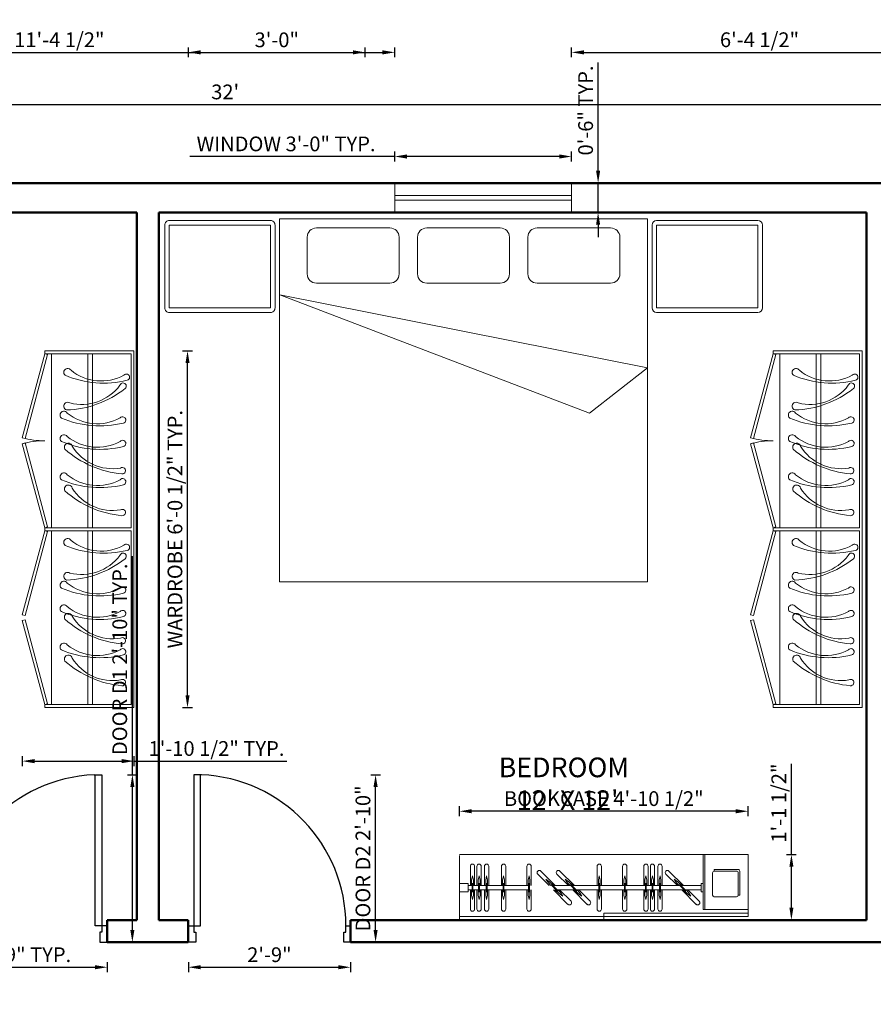
# Model space of a CAD drawing. Units: inches. Extents: x 1961 to 3038, y 800 to 1438.
# Tile 12 of 13: x 2775 to 2949, y 1148 to 1348. Entities that reach past the tile are written whole.
import ezdxf

# ---------------------------------------------------------------- set-up
doc = ezdxf.new("R2010")
doc.units = ezdxf.units.IN
for name, color, linetype, lineweight in [('A-ANNO-DIMS', 2, 'Continuous', 18), ('A-AREA-IDEN', 7, 'Continuous', 25), ('A-DOOR', 3, 'Continuous', 25), ('A-FURN', 8, 'Continuous', 18), ('A-GLAZ', 4, 'Continuous', 18), ('A-WALL', 7, 'Continuous', 50)]:
    doc.layers.add(name, color=color, linetype=linetype, lineweight=lineweight)
doc.styles.get("Standard").update_dxf_attribs({"font": 'arial.ttf'})
doc.dimstyles.new('ISO-25', dxfattribs={"dimtxt": 3, "dimasz": 2.5, "dimexe": 1, "dimexo": 1, "dimtad": 1, "dimdec": 4, "dimlunit": 4, "dimtxsty": 'Standard', "dimcen": 2.5, "dimadec": 0, "dimazin": 0, "dimtfac": 1, "dimtdec": 4, "dimtmove": 0, "dimatfit": 3, "dimfxl": 1, "dimfxlon": 1, "dimarcsym": 0})

# ---------------------------------------------------------------- blocks, each defined once
blk = doc.blocks.new('door 29')
for p, q in [((2811.91, 1194.49), (2810.4, 1194.49)), ((2810.4, 1194.49), (2810.4, 1163.76)), ((2811.74, 1163.76), (2811.74, 1194.49)), ((2809.27, 1163.76), (2811.74, 1163.76)), ((2810.4, 1163.76), (2810.4, 1162.42)), ((2810.4, 1162.42), (2810.81, 1162.42)), ((2810.81, 1162.42), (2810.81, 1160.42)), ((2810.81, 1160.42), (2809.27, 1160.42))]:
    blk.add_line(p, q)
blk.add_lwpolyline([(2842.27, 1160.42), (2840.93, 1160.42), (2840.93, 1162.42), (2841.34, 1162.42), (2841.34, 1163.76), (2842.27, 1163.76)])
blk.add_arc((2810.58, 1163.76), 30.76, 0, 87.5104)
blk = doc.blocks.new('A$C793B20D3')
for p, q in [((0.575, 1.9405), (0.025, 1.9405)), ((0.025, 1.9405), (0.025, 1.4905)), ((0.575, 1.4905), (0.575, 1.9405)), ((0.625, 0), (0.625, 1.975)), ((2.625, 1.975), (0.625, 1.975)), ((2.625, 0), (2.625, 1.975)), ((2.65, 1.4905), (2.65, 1.9405)), ((2.675, 1.9655), (3.225, 1.9655)), ((3.25, 1.9405), (3.25, 1.4905)), ((0.775, 1.675), (0.775, 1.875)), ((0.825, 1.925), (1.225, 1.925)), ((1.275, 1.675), (1.275, 1.875)), ((1.375, 1.675), (1.375, 1.875)), ((1.425, 1.925), (1.825, 1.925)), ((1.875, 1.675), (1.875, 1.875)), ((1.975, 1.675), (1.975, 1.875)), ((2.025, 1.925), (2.425, 1.925)), ((2.475, 1.675), (2.475, 1.875)), ((0.825, 1.625), (1.225, 1.625)), ((1.425, 1.625), (1.825, 1.625)), ((2.025, 1.625), (2.425, 1.625)), ((0.6256, 1.5604), (2.3107, 0.9169)), ((0.6256, 1.5604), (2.625, 1.1646)), ((0.025, 1.4905), (0.575, 1.4905)), ((3.225, 1.4655), (2.675, 1.4655)), ((2.3107, 0.9169), (2.625, 1.1646)), ((2.625, 0), (0.625, 0))]:
    blk.add_line(p, q)
at = {"flags": 128}
blk.add_lwpolyline([(0, 1.9405), (0, 1.4905, 0.414214), (0.025, 1.4655), (0.575, 1.4655, 0.414214), (0.6, 1.4905), (0.6, 1.9405, 0.414214), (0.575, 1.9655), (0.025, 1.9655, 0.414214)], format="xyb", close=True, dxfattribs=at)
blk.add_lwpolyline([(3.225, 1.9405), (3.225, 1.4905), (2.675, 1.4905), (2.675, 1.9405)], close=True)
for centre, radius, start, end in [((2.675, 1.9405), 0.025, 90, 180), ((3.225, 1.9405), 0.025, 0, 90), ((0.825, 1.875), 0.05, 90, 180), ((1.225, 1.875), 0.05, 0, 90), ((1.425, 1.875), 0.05, 90, 180), ((1.825, 1.875), 0.05, 0, 90), ((2.025, 1.875), 0.05, 90, 180), ((2.425, 1.875), 0.05, 0, 90), ((0.825, 1.675), 0.05, 180, 270), ((1.225, 1.675), 0.05, 270, 0), ((1.425, 1.675), 0.05, 180, 270), ((1.825, 1.675), 0.05, 270, 0), ((2.025, 1.675), 0.05, 180, 270), ((2.425, 1.675), 0.05, 270, 0), ((2.675, 1.4905), 0.025, 180, 270), ((3.225, 1.4905), 0.025, 270, 0)]:
    blk.add_arc(centre, radius, start, end)
blk = doc.blocks.new('A$C41DA168A')
for p, q in [((151.4, 2380), (151.4, 2400)), ((151.4, 2400), (751.4, 2400)), ((751.4, 2400), (751.4, 0)), ((151.4, 2380), (0, 1814.9)), ((19.3, 1809.8), (170.7, 2374.8)), ((731.4, 2380), (151.4, 2380)), ((170.7, 2374.8), (151.4, 2380)), ((196.6, 1210), (196.6, 2380)), ((441.4, 1210), (441.4, 2380)), ((471.4, 1210), (471.4, 2380)), ((731.4, 1210), (731.4, 2380)), ((0, 1814.9), (19.3, 1809.8)), ((0, 1775.1), (19.3, 1780.2)), ((151.4, 1210), (0, 1775.1)), ((19.3, 1780.2), (170.7, 1215.2)), ((170.7, 1215.2), (151.4, 1210)), ((151.4, 1210), (731.4, 1210)), ((151.4, 1190), (151.4, 1210)), ((151.4, 1190), (0, 624.9)), ((19.3, 619.8), (170.7, 1184.8)), ((731.4, 1190), (151.4, 1190)), ((170.7, 1184.8), (151.4, 1190)), ((196.6, 20), (196.6, 1190)), ((441.4, 1190), (441.4, 20)), ((471.4, 1190), (471.4, 20)), ((731.4, 20), (731.4, 1190)), ((0, 624.9), (19.3, 619.8)), ((0, 585.1), (19.3, 590.2)), ((151.4, 20), (0, 585.1)), ((19.3, 590.2), (170.7, 25.2)), ((170.7, 25.2), (151.4, 20)), ((151.4, 0), (151.4, 20)), ((151.4, 20), (731.4, 20)), ((751.4, 0), (151.4, 0))]:
    blk.add_line(p, q)
for centre, radius, start, end in [((305.7, 2255.1), 26.3, 32.27517, 228.96506), ((530.9, 2518.7), 321.7, 230.8748, 298.39865), ((548.2, 2849.7), 667, 247.08357, 283.63935), ((700.5, 2222.3), 21.4, 283.29422, 141.17028), ((277.3, 2668.9), 667, 271.7885, 308.34429), ((399.9, 2361), 321.7, 255.57974, 323.10358), ((677.9, 2162.6), 21.4, 307.99916, 165.87521), ((305.5, 2027.4), 26.3, 56.9801, 253.67), ((280.2, 1967.6), 26.3, 32.27517, 228.96506), ((522.6, 2562.2), 667, 247.08357, 283.63935), ((505.3, 2231.2), 321.7, 230.8748, 298.39865), ((675, 1934.8), 21.4, 283.29422, 141.17028), ((151.4, 2380), 585, 255, 270), ((151.4, 1210), 585, 90, 105), ((280.2, 1809.7), 26.3, 32.27517, 228.96506), ((522.6, 2404.2), 667, 247.08357, 283.63935), ((505.3, 2073.2), 321.7, 230.8748, 298.39865), ((675, 1776.9), 21.4, 283.29422, 141.17028), ((309.6, 1752), 26.3, 13.45499, 210.14489), ((730.9, 2236.5), 667, 228.26339, 264.81917), ((607.8, 1928.8), 321.7, 212.05463, 279.57847), ((672.7, 1593.6), 21.4, 264.47404, 122.3501), ((280.2, 1552.2), 26.3, 32.27517, 228.96506), ((522.6, 2146.7), 667, 247.08357, 283.63935), ((505.3, 1815.7), 321.7, 230.8748, 298.39865), ((675, 1519.4), 21.4, 283.29422, 141.17028), ((309.6, 1470.8), 26.3, 13.45499, 210.14489), ((730.9, 1955.3), 667, 228.26339, 264.81917), ((607.8, 1647.6), 321.7, 212.05463, 279.57847), ((672.7, 1312.3), 21.4, 264.47404, 122.3501), ((305.7, 1111), 26.3, 32.27517, 228.96506), ((548.2, 1705.5), 667, 247.08357, 283.63935), ((530.9, 1374.6), 321.7, 230.8748, 298.39865), ((700.5, 1078.2), 21.4, 283.29422, 141.17028), ((277.3, 1524.8), 667, 271.7885, 308.34429), ((399.9, 1216.9), 321.7, 255.57974, 323.10358), ((677.9, 1018.5), 21.4, 307.99916, 165.87521), ((305.5, 883.3), 26.3, 56.9801, 253.67), ((280.2, 823.5), 26.3, 32.27517, 228.96506), ((522.6, 1418), 667, 247.08357, 283.63935), ((505.3, 1087.1), 321.7, 230.8748, 298.39865), ((675, 790.7), 21.4, 283.29422, 141.17028), ((280.2, 665.6), 26.3, 32.27517, 228.96506), ((505.3, 929.1), 321.7, 230.8748, 298.39865), ((522.6, 1260.1), 667, 247.08357, 283.63935), ((309.6, 607.9), 26.3, 13.45499, 210.14489), ((607.8, 784.7), 321.7, 212.05463, 279.57847), ((675, 632.8), 21.4, 283.29422, 141.17028), ((730.9, 1092.4), 667, 228.26339, 264.81917), ((672.7, 449.5), 21.4, 264.47404, 122.3501), ((280.2, 408.1), 26.3, 32.27517, 228.96506), ((505.3, 671.6), 321.7, 230.8748, 298.39865), ((522.6, 1002.6), 667, 247.08357, 283.63935), ((309.6, 326.7), 26.3, 13.45499, 210.14489), ((607.8, 503.5), 321.7, 212.05463, 279.57847), ((675, 375.3), 21.4, 283.29422, 141.17028), ((730.9, 811.2), 667, 228.26339, 264.81917), ((672.7, 168.2), 21.4, 264.47404, 122.3501)]:
    blk.add_arc(centre, radius, start, end)
blk = doc.blocks.new('A$C58C54B33')
for p, q in [((0, 3374), (0, 1687)), ((756, 3374), (0, 3374)), ((40, 3374), (40, 0)), ((428, 3374), (328, 3374)), ((328, 3274), (328, 3374)), ((428, 3274), (428, 3374)), ((766, 3374), (766, 0)), ((353, 3247), (128, 3247)), ((239, 3222), (289, 3233)), ((289, 3233), (353, 3233)), ((428, 3274), (328, 3274)), ((428, 3227), (328, 3227)), ((328, 3217), (328, 3227)), ((353, 3150), (353, 3274)), ((403, 3150), (403, 3274)), ((628, 3247), (403, 3247)), ((403, 3233), (467, 3233)), ((428, 3217), (428, 3227)), ((517, 3222), (467, 3233)), ((353, 3197), (128, 3197)), ((353, 3170), (128, 3170)), ((353, 3120), (128, 3120)), ((239, 3222), (289, 3211)), ((239, 3145), (289, 3156)), ((239, 3145), (289, 3134)), ((353, 3211), (289, 3211)), ((289, 3156), (353, 3156)), ((353, 3134), (289, 3134)), ((428, 3217), (328, 3217)), ((428, 3150), (328, 3150)), ((328, 3140), (328, 3150)), ((428, 3140), (328, 3140)), ((353, 3217), (353, 3150)), ((353, 3140), (353, 3062)), ((403, 3217), (403, 3150)), ((467, 3211), (403, 3211)), ((628, 3197), (403, 3197)), ((628, 3170), (403, 3170)), ((403, 3156), (467, 3156)), ((403, 3140), (403, 3062)), ((467, 3134), (403, 3134)), ((628, 3120), (403, 3120)), ((428, 3140), (428, 3150)), ((517, 3222), (467, 3211)), ((517, 3145), (467, 3156)), ((517, 3145), (467, 3134)), ((353, 3082), (128, 3082)), ((353, 3032), (128, 3032)), ((239, 3057), (289, 3068)), ((239, 3057), (289, 3046)), ((289, 3068), (353, 3068)), ((353, 3046), (289, 3046)), ((428, 3062), (328, 3062)), ((328, 3052), (328, 3062)), ((428, 3052), (328, 3052)), ((353, 3052), (353, 2864)), ((628, 3082), (403, 3082)), ((403, 3068), (467, 3068)), ((403, 3052), (403, 2864)), ((467, 3046), (403, 3046)), ((628, 3032), (403, 3032)), ((428, 3052), (428, 3062)), ((517, 3057), (467, 3068)), ((517, 3057), (467, 3046)), ((353, 2884), (128, 2884)), ((628, 2884), (403, 2884)), ((353, 2834), (128, 2834)), ((239, 2859), (289, 2870)), ((239, 2859), (289, 2848)), ((289, 2870), (353, 2870)), ((353, 2848), (289, 2848)), ((428, 2864), (328, 2864)), ((328, 2854), (328, 2864)), ((428, 2854), (328, 2854)), ((353, 2854), (353, 2566)), ((403, 2870), (467, 2870)), ((403, 2854), (403, 2566)), ((467, 2848), (403, 2848)), ((628, 2834), (403, 2834)), ((428, 2854), (428, 2864)), ((517, 2859), (467, 2870)), ((517, 2859), (467, 2848)), ((353, 2586), (128, 2586)), ((353, 2536), (128, 2536)), ((239, 2561), (289, 2572)), ((239, 2561), (289, 2550)), ((289, 2572), (353, 2572)), ((353, 2550), (289, 2550)), ((328, 2556), (328, 2566)), ((428, 2566), (328, 2566)), ((428, 2556), (328, 2556)), ((628, 2586), (403, 2586)), ((403, 2572), (467, 2572)), ((467, 2550), (403, 2550)), ((628, 2536), (403, 2536)), ((428, 2556), (428, 2566)), ((517, 2561), (467, 2572)), ((517, 2561), (467, 2550)), ((537, 2459), (403, 2325)), ((572, 2424), (403, 2254)), ((410, 2304), (339, 2233)), ((403, 2305), (433, 2335)), ((448, 2320), (403, 2274)), ((417, 2296), (410, 2304)), ((476, 2363), (433, 2335)), ((476, 2363), (448, 2320)), ((353, 2275), (183, 2106)), ((353, 2204), (219, 2070)), ((280, 2167), (308, 2210)), ((280, 2167), (323, 2194)), ((308, 2210), (353, 2255)), ((353, 2224), (323, 2194)), ((346, 2226), (339, 2233)), ((417, 2296), (346, 2226)), ((353, 2233), (353, 2022)), ((403, 2283), (403, 2072)), ((537, 2235), (403, 2101)), ((572, 2200), (403, 2030)), ((410, 2079), (339, 2009)), ((417, 2072), (346, 2002)), ((403, 2081), (433, 2111)), ((448, 2095), (403, 2050)), ((417, 2072), (410, 2079)), ((476, 2138), (433, 2111)), ((476, 2138), (448, 2095)), ((353, 2051), (183, 1881)), ((353, 1980), (219, 1846)), ((280, 1942), (308, 1985)), ((280, 1942), (323, 1970)), ((308, 1985), (353, 2031)), ((353, 2000), (323, 1970)), ((346, 2002), (339, 2009)), ((353, 1745), (353, 2008)), ((403, 1745), (403, 2058)), ((353, 1765), (128, 1765)), ((239, 1740), (289, 1751)), ((239, 1740), (289, 1729)), ((289, 1751), (353, 1751)), ((353, 1729), (289, 1729)), ((428, 1745), (328, 1745)), ((328, 1735), (328, 1745)), ((428, 1735), (328, 1735)), ((353, 1735), (353, 1447)), ((628, 1765), (403, 1765)), ((403, 1751), (467, 1751)), ((403, 1735), (403, 1447)), ((467, 1729), (403, 1729)), ((428, 1735), (428, 1745)), ((517, 1740), (467, 1751)), ((517, 1740), (467, 1729)), ((0, 1687), (80, 1687)), ((80, 1687), (80, 0)), ((353, 1715), (128, 1715)), ((628, 1715), (403, 1715)), ((353, 1467), (128, 1467)), ((353, 1417), (128, 1417)), ((239, 1442), (289, 1453)), ((239, 1442), (289, 1431)), ((289, 1453), (353, 1453)), ((353, 1431), (289, 1431)), ((328, 1437), (328, 1447)), ((428, 1447), (328, 1447)), ((428, 1437), (328, 1437)), ((353, 1123), (353, 1437)), ((628, 1467), (403, 1467)), ((403, 1453), (467, 1453)), ((403, 1123), (403, 1437)), ((467, 1431), (403, 1431)), ((628, 1417), (403, 1417)), ((428, 1437), (428, 1447)), ((517, 1442), (467, 1453)), ((517, 1442), (467, 1431)), ((353, 1220), (128, 1220)), ((353, 1170), (128, 1170)), ((239, 1195), (289, 1206)), ((239, 1195), (289, 1184)), ((289, 1206), (353, 1206)), ((353, 1184), (289, 1184)), ((428, 1200), (328, 1200)), ((328, 1190), (328, 1200)), ((428, 1190), (328, 1190)), ((353, 1190), (353, 1123)), ((628, 1220), (403, 1220)), ((403, 1206), (467, 1206)), ((403, 1190), (403, 1123)), ((467, 1184), (403, 1184)), ((628, 1170), (403, 1170)), ((428, 1190), (428, 1200)), ((517, 1195), (467, 1206)), ((517, 1195), (467, 1184)), ((353, 1143), (128, 1143)), ((353, 1093), (128, 1093)), ((353, 1055), (128, 1055)), ((239, 1118), (289, 1129)), ((239, 1118), (289, 1107)), ((239, 1030), (289, 1041)), ((289, 1129), (353, 1129)), ((353, 1107), (289, 1107)), ((289, 1041), (353, 1041)), ((428, 1123), (328, 1123)), ((328, 1113), (328, 1123)), ((428, 1113), (328, 1113)), ((353, 1113), (353, 1035)), ((628, 1143), (403, 1143)), ((403, 1129), (467, 1129)), ((403, 1113), (403, 1035)), ((467, 1107), (403, 1107)), ((628, 1093), (403, 1093)), ((628, 1055), (403, 1055)), ((403, 1041), (467, 1041)), ((428, 1113), (428, 1123)), ((517, 1118), (467, 1129)), ((517, 1118), (467, 1107)), ((517, 1030), (467, 1041)), ((353, 1005), (128, 1005)), ((239, 1030), (289, 1019)), ((353, 1019), (289, 1019)), ((428, 1035), (328, 1035)), ((328, 1025), (328, 1035)), ((428, 1025), (328, 1025)), ((353, 1025), (353, 748)), ((403, 1025), (403, 798)), ((467, 1019), (403, 1019)), ((628, 1005), (403, 1005)), ((537, 961), (403, 826)), ((572, 925), (403, 756)), ((428, 1025), (428, 1035)), ((517, 1030), (467, 1019)), ((403, 807), (433, 836)), ((448, 821), (403, 776)), ((476, 864), (433, 836)), ((476, 864), (448, 821)), ((353, 776), (183, 607)), ((353, 706), (219, 572)), ((280, 668), (308, 711)), ((280, 668), (323, 696)), ((308, 711), (353, 757)), ((353, 726), (323, 696)), ((410, 805), (339, 734)), ((346, 727), (339, 734)), ((417, 798), (346, 727)), ((353, 550), (353, 734)), ((403, 550), (403, 784)), ((417, 798), (410, 805)), ((766, 525), (123, 525)), ((123, 525), (123, 0)), ((766, 505), (123, 505)), ((428, 550), (328, 550)), ((328, 550), (328, 525)), ((428, 550), (428, 525)), ((272, 136), (272, 396)), ((292, 416), (552, 416)), ((572, 398), (591, 398)), ((572, 396), (572, 136)), ((591, 398), (591, 118)), ((291, 98), (291, 116)), ((552, 116), (292, 116)), ((40, 0), (766, 0)), ((571, 98), (291, 98))]:
    blk.add_line(p, q)
for centre, radius, start, end in [((128, 3222), 25, 90, 270), ((628, 3222), 25, 270, 90), ((128, 3145), 25, 90, 270), ((628, 3145), 25, 270, 90), ((128, 3057), 25, 90, 270), ((628, 3057), 25, 270, 90), ((128, 2859), 25, 90, 270), ((628, 2859), 25, 270, 90), ((128, 2561), 25, 90, 270), ((628, 2561), 25, 270, 90), ((555, 2441), 25, 315, 135), ((555, 2217), 25, 315, 135), ((201, 2088), 25, 135, 315), ((201, 1864), 25, 135, 315), ((128, 1740), 25, 90, 270), ((628, 1740), 25, 270, 90), ((128, 1442), 25, 90, 270), ((628, 1442), 25, 270, 90), ((128, 1195), 25, 90, 270), ((628, 1195), 25, 270, 90), ((128, 1118), 25, 90, 270), ((128, 1030), 25, 90, 270), ((628, 1118), 25, 270, 90), ((628, 1030), 25, 270, 90), ((555, 943), 25, 315, 135), ((201, 589), 25, 135, 315), ((292, 396), 20, 90, 180), ((552, 396), 20, 0, 90), ((292, 136), 20, 180, 270), ((552, 136), 20, 270, 0), ((571, 118), 20, 270, 0)]:
    blk.add_arc(centre, radius, start, end)
blk = doc.blocks.new('*D25')
at = {"layer": 'A-ANNO-DIMS', "color": 0, "lineweight": -2, "transparency": 16777216}
for p, q in [((2624.77, 1329.92), (2624.77, 1331.92)), ((2627.27, 1330.92), (3006.27, 1330.92)), ((3008.77, 1329.92), (3008.77, 1331.92))]:
    blk.add_line(p, q, dxfattribs=at)
at = {"layer": 'A-ANNO-DIMS', "color": 0, "transparency": 16777216}
for points in [[(2627.27, 1331.34), (2627.27, 1330.51), (2624.77, 1330.92)], [(3006.27, 1331.34), (3006.27, 1330.51), (3008.77, 1330.92)]]:
    blk.add_solid(points, dxfattribs=at)
at = {"layer": 'Defpoints', "color": 0, "transparency": 16777216}
for p in [(3008.77, 1330.92), (2624.77, 1314.92), (3008.77, 1314.92)]:
    blk.add_point(p, dxfattribs=at)
at = {"layer": 'A-ANNO-DIMS', "color": 0, "transparency": 16777216, "insert": (2816.77, 1333.08), "char_height": 3, "attachment_point": 5}
blk.add_mtext("32'", dxfattribs=at)
blk = doc.blocks.new('WIN-36IN')
for p, q in [((0, 36), (6, 36)), ((2.5, 36), (2.5, 0)), ((3.5, 36), (3.5, 0)), ((0, 0), (6, 0))]:
    blk.add_line(p, q)
blk = doc.blocks.new('DOOR-SWING-33IN')
for p, q in [((30.36, 34.07), (31.87, 34.07)), ((30.53, 3.34), (30.53, 34.07)), ((31.87, 34.07), (31.87, 3.34)), ((33, 3.34), (30.53, 3.34)), ((31.87, 2), (31.46, 2)), ((31.46, 2), (31.46, 0)), ((31.87, 3.34), (31.87, 2)), ((31.46, 0), (33, 0))]:
    blk.add_line(p, q)
blk.add_lwpolyline([(0, 0), (1.34, 0), (1.34, 2), (0.93, 2), (0.93, 3.34), (0, 3.34)])
blk.add_arc((31.69, 3.34), 30.76, 92.4896, 180)
blk = doc.blocks.new('*D31')
at = {"layer": 'A-ANNO-DIMS', "color": 0, "lineweight": -2, "transparency": 16777216}
for p, q in [((2808.1, 1280.77), (2810.1, 1280.77)), ((2809.1, 1210.65), (2809.1, 1278.27)), ((2808.1, 1208.15), (2810.1, 1208.15))]:
    blk.add_line(p, q, dxfattribs=at)
at = {"layer": 'A-ANNO-DIMS', "color": 0, "transparency": 16777216}
for points in [[(2808.69, 1278.27), (2809.52, 1278.27), (2809.1, 1280.77)], [(2808.69, 1210.65), (2809.52, 1210.65), (2809.1, 1208.15)]]:
    blk.add_solid(points, dxfattribs=at)
at = {"layer": 'Defpoints', "color": 0, "transparency": 16777216}
for p in [(2798.21, 1280.77), (2809.1, 1280.77), (2798.21, 1208.15)]:
    blk.add_point(p, dxfattribs=at)
at = {"layer": 'A-ANNO-DIMS', "color": 0, "transparency": 16777216, "insert": (2806.93, 1244.46), "char_height": 3, "attachment_point": 5, "rotation": 90}
blk.add_mtext('WARDROBE 6\'-0 1/2" TYP.', dxfattribs=at)
blk = doc.blocks.new('*D32')
at = {"layer": 'A-ANNO-DIMS', "color": 0, "lineweight": -2, "transparency": 16777216}
for p, q in [((2775.47, 1198.26), (2775.47, 1196.26)), ((2777.97, 1197.26), (2795.71, 1197.26)), ((2798.21, 1198.26), (2798.21, 1196.26)), ((2798.21, 1197.26), (2829.29, 1197.26))]:
    blk.add_line(p, q, dxfattribs=at)
at = {"layer": 'A-ANNO-DIMS', "color": 0, "transparency": 16777216}
for points in [[(2777.97, 1197.68), (2777.97, 1196.84), (2775.47, 1197.26)], [(2795.71, 1197.68), (2795.71, 1196.84), (2798.21, 1197.26)]]:
    blk.add_solid(points, dxfattribs=at)
at = {"layer": 'Defpoints', "color": 0, "transparency": 16777216}
for p in [(2775.47, 1208.15), (2798.21, 1208.15), (2798.21, 1197.26)]:
    blk.add_point(p, dxfattribs=at)
at = {"layer": 'A-ANNO-DIMS', "color": 0, "transparency": 16777216, "insert": (2815, 1199.44), "char_height": 3, "attachment_point": 5}
blk.add_mtext('1\'-10 1/2" TYP.', dxfattribs=at)
blk = doc.blocks.new('*D33')
at = {"layer": 'A-ANNO-DIMS', "color": 0, "lineweight": -2, "transparency": 16777216}
for p, q in [((2851.27, 1319.32), (2851.27, 1321.32)), ((2887.27, 1319.32), (2887.27, 1321.32)), ((2851.27, 1320.32), (2809.56, 1320.32)), ((2884.77, 1320.32), (2853.77, 1320.32))]:
    blk.add_line(p, q, dxfattribs=at)
at = {"layer": 'A-ANNO-DIMS', "color": 0, "transparency": 16777216}
for points in [[(2853.77, 1320.74), (2853.77, 1319.9), (2851.27, 1320.32)], [(2884.77, 1320.74), (2884.77, 1319.9), (2887.27, 1320.32)]]:
    blk.add_solid(points, dxfattribs=at)
at = {"layer": 'Defpoints', "color": 0, "transparency": 16777216}
for p in [(2851.27, 1320.32), (2851.27, 1314.92), (2887.27, 1314.92)]:
    blk.add_point(p, dxfattribs=at)
at = {"layer": 'A-ANNO-DIMS', "color": 0, "transparency": 16777216, "insert": (2829.16, 1322.5), "char_height": 3, "attachment_point": 5}
blk.add_mtext('WINDOW 3\'-0" TYP.', dxfattribs=at)
blk = doc.blocks.new('*D34')
at = {"layer": 'A-ANNO-DIMS', "color": 0, "lineweight": -2, "transparency": 16777216}
for p, q in [((2892.67, 1317.42), (2892.67, 1339.46)), ((2891.67, 1314.92), (2893.67, 1314.92)), ((2892.67, 1308.92), (2892.67, 1314.92)), ((2891.67, 1308.92), (2893.67, 1308.92)), ((2892.67, 1306.42), (2892.67, 1303.92))]:
    blk.add_line(p, q, dxfattribs=at)
at = {"layer": 'A-ANNO-DIMS', "color": 0, "transparency": 16777216}
for points in [[(2892.25, 1317.42), (2893.08, 1317.42), (2892.67, 1314.92)], [(2892.25, 1306.42), (2893.08, 1306.42), (2892.67, 1308.92)]]:
    blk.add_solid(points, dxfattribs=at)
at = {"layer": 'Defpoints', "color": 0, "transparency": 16777216}
for p in [(2887.27, 1314.92), (2892.67, 1314.92), (2887.27, 1308.92)]:
    blk.add_point(p, dxfattribs=at)
at = {"layer": 'A-ANNO-DIMS', "color": 0, "transparency": 16777216, "insert": (2890.51, 1329.69), "char_height": 3, "attachment_point": 5, "rotation": 90}
blk.add_mtext('0\'-6" TYP.', dxfattribs=at)
blk = doc.blocks.new('*D47')
at = {"layer": 'A-ANNO-DIMS', "color": 0, "lineweight": -2, "transparency": 16777216}
for p, q in [((2797.88, 1194.49), (2797.88, 1238.97)), ((2796.88, 1194.49), (2798.88, 1194.49)), ((2797.88, 1162.92), (2797.88, 1191.99)), ((2796.88, 1160.42), (2798.88, 1160.42))]:
    blk.add_line(p, q, dxfattribs=at)
at = {"layer": 'A-ANNO-DIMS', "color": 0, "transparency": 16777216}
for points in [[(2797.46, 1191.99), (2798.3, 1191.99), (2797.88, 1194.49)], [(2797.46, 1162.92), (2798.3, 1162.92), (2797.88, 1160.42)]]:
    blk.add_solid(points, dxfattribs=at)
at = {"layer": 'Defpoints', "color": 0, "transparency": 16777216}
for p in [(2792.77, 1194.49), (2797.88, 1194.49), (2792.77, 1160.42)]:
    blk.add_point(p, dxfattribs=at)
at = {"layer": 'A-ANNO-DIMS', "color": 0, "transparency": 16777216, "insert": (2795.7, 1217.98), "char_height": 3, "attachment_point": 5, "rotation": 90}
blk.add_mtext('DOOR D1 2\'-10" TYP.', dxfattribs=at)
blk = doc.blocks.new('*D48')
at = {"layer": 'A-ANNO-DIMS', "color": 0, "lineweight": -2, "transparency": 16777216}
for p, q in [((2759.77, 1156.31), (2759.77, 1154.31)), ((2762.27, 1155.31), (2790.27, 1155.31)), ((2792.77, 1156.31), (2792.77, 1154.31))]:
    blk.add_line(p, q, dxfattribs=at)
at = {"layer": 'A-ANNO-DIMS', "color": 0, "transparency": 16777216}
for points in [[(2762.27, 1155.73), (2762.27, 1154.89), (2759.77, 1155.31)], [(2790.27, 1155.73), (2790.27, 1154.89), (2792.77, 1155.31)]]:
    blk.add_solid(points, dxfattribs=at)
at = {"layer": 'Defpoints', "color": 0, "transparency": 16777216}
for p in [(2759.77, 1160.42), (2792.77, 1160.42), (2792.77, 1155.31)]:
    blk.add_point(p, dxfattribs=at)
at = {"layer": 'A-ANNO-DIMS', "color": 0, "transparency": 16777216, "insert": (2776.27, 1157.47), "char_height": 3, "attachment_point": 5}
blk.add_mtext('2\'-9" TYP.', dxfattribs=at)
blk = doc.blocks.new('*D49')
at = {"layer": 'A-ANNO-DIMS', "color": 0, "lineweight": -2, "transparency": 16777216}
for p, q in [((2846.38, 1194.49), (2848.38, 1194.49)), ((2847.38, 1162.92), (2847.38, 1191.99)), ((2846.38, 1160.42), (2848.38, 1160.42))]:
    blk.add_line(p, q, dxfattribs=at)
at = {"layer": 'A-ANNO-DIMS', "color": 0, "transparency": 16777216}
for points in [[(2846.96, 1191.99), (2847.8, 1191.99), (2847.38, 1194.49)], [(2846.96, 1162.92), (2847.8, 1162.92), (2847.38, 1160.42)]]:
    blk.add_solid(points, dxfattribs=at)
at = {"layer": 'Defpoints', "color": 0, "transparency": 16777216}
for p in [(2842.27, 1194.49), (2847.38, 1194.49), (2842.27, 1160.42)]:
    blk.add_point(p, dxfattribs=at)
at = {"layer": 'A-ANNO-DIMS', "color": 0, "transparency": 16777216, "insert": (2845.2, 1177.46), "char_height": 3, "attachment_point": 5, "rotation": 90}
blk.add_mtext('DOOR D2 2\'-10"', dxfattribs=at)
blk = doc.blocks.new('*D50')
at = {"layer": 'A-ANNO-DIMS', "color": 0, "lineweight": -2, "transparency": 16777216}
for p, q in [((2809.27, 1156.31), (2809.27, 1154.31)), ((2811.77, 1155.31), (2839.77, 1155.31)), ((2842.27, 1156.31), (2842.27, 1154.31))]:
    blk.add_line(p, q, dxfattribs=at)
at = {"layer": 'A-ANNO-DIMS', "color": 0, "transparency": 16777216}
for points in [[(2811.77, 1155.73), (2811.77, 1154.89), (2809.27, 1155.31)], [(2839.77, 1155.73), (2839.77, 1154.89), (2842.27, 1155.31)]]:
    blk.add_solid(points, dxfattribs=at)
at = {"layer": 'Defpoints', "color": 0, "transparency": 16777216}
for p in [(2809.27, 1160.42), (2842.27, 1160.42), (2842.27, 1155.31)]:
    blk.add_point(p, dxfattribs=at)
at = {"layer": 'A-ANNO-DIMS', "color": 0, "transparency": 16777216, "insert": (2825.77, 1157.47), "char_height": 3, "attachment_point": 5}
blk.add_mtext('2\'-9"', dxfattribs=at)
blk = doc.blocks.new('*D53')
at = {"layer": 'A-ANNO-DIMS', "color": 0, "lineweight": -2, "transparency": 16777216}
for p, q in [((2864.46, 1186.06), (2864.46, 1188.06)), ((2920.7, 1187.06), (2866.96, 1187.06)), ((2923.2, 1186.06), (2923.2, 1188.06))]:
    blk.add_line(p, q, dxfattribs=at)
at = {"layer": 'A-ANNO-DIMS', "color": 0, "transparency": 16777216}
for points in [[(2866.96, 1187.48), (2866.96, 1186.64), (2864.46, 1187.06)], [(2920.7, 1187.48), (2920.7, 1186.64), (2923.2, 1187.06)]]:
    blk.add_solid(points, dxfattribs=at)
at = {"layer": 'Defpoints', "color": 0, "transparency": 16777216}
for p in [(2864.46, 1187.06), (2864.46, 1178.25), (2923.2, 1178.25)]:
    blk.add_point(p, dxfattribs=at)
at = {"layer": 'A-ANNO-DIMS', "color": 0, "transparency": 16777216, "insert": (2893.83, 1189.24), "char_height": 3, "attachment_point": 5}
blk.add_mtext('BOOKCASE 4\'-10 1/2"', dxfattribs=at)
blk = doc.blocks.new('*D54')
at = {"layer": 'A-ANNO-DIMS', "color": 0, "lineweight": -2, "transparency": 16777216}
for p, q in [((2932.01, 1178.25), (2932.01, 1196.68)), ((2931.01, 1178.25), (2933.01, 1178.25)), ((2932.01, 1167.42), (2932.01, 1175.75)), ((2931.01, 1164.92), (2933.01, 1164.92))]:
    blk.add_line(p, q, dxfattribs=at)
at = {"layer": 'A-ANNO-DIMS', "color": 0, "transparency": 16777216}
for points in [[(2931.6, 1175.75), (2932.43, 1175.75), (2932.01, 1178.25)], [(2931.6, 1167.42), (2932.43, 1167.42), (2932.01, 1164.92)]]:
    blk.add_solid(points, dxfattribs=at)
at = {"layer": 'Defpoints', "color": 0, "transparency": 16777216}
for p in [(2923.2, 1178.25), (2932.01, 1178.25), (2923.2, 1164.92)]:
    blk.add_point(p, dxfattribs=at)
at = {"layer": 'A-ANNO-DIMS', "color": 0, "transparency": 16777216, "insert": (2929.84, 1188.72), "char_height": 3, "attachment_point": 5, "rotation": 90}
blk.add_mtext('1\'-1 1/2"', dxfattribs=at)
blk = doc.blocks.new('*D75')
at = {"layer": 'A-ANNO-DIMS', "color": 0, "lineweight": -2, "transparency": 16777216}
for p, q in [((2809.27, 1340.52), (2809.27, 1342.52)), ((2811.77, 1341.52), (2842.77, 1341.52)), ((2845.27, 1340.52), (2845.27, 1342.52))]:
    blk.add_line(p, q, dxfattribs=at)
at = {"layer": 'A-ANNO-DIMS', "color": 0, "transparency": 16777216}
for points in [[(2811.77, 1341.94), (2811.77, 1341.1), (2809.27, 1341.52)], [(2842.77, 1341.94), (2842.77, 1341.1), (2845.27, 1341.52)]]:
    blk.add_solid(points, dxfattribs=at)
at = {"layer": 'Defpoints', "color": 0, "transparency": 16777216}
for p in [(2845.27, 1341.52), (2809.27, 970.92), (2845.27, 970.92)]:
    blk.add_point(p, dxfattribs=at)
at = {"layer": 'A-ANNO-DIMS', "color": 0, "transparency": 16777216, "insert": (2827.27, 1343.68), "char_height": 3, "attachment_point": 5}
blk.add_mtext('3\'-0"', dxfattribs=at)
blk = doc.blocks.new('*D77')
at = {"layer": 'A-ANNO-DIMS', "color": 0, "lineweight": -2, "transparency": 16777216}
for p, q in [((2714.77, 1340.52), (2714.77, 1342.52)), ((2717.27, 1341.52), (2848.77, 1341.52)), ((2851.27, 1340.52), (2851.27, 1342.52))]:
    blk.add_line(p, q, dxfattribs=at)
at = {"layer": 'A-ANNO-DIMS', "color": 0, "transparency": 16777216}
for points in [[(2717.27, 1341.94), (2717.27, 1341.1), (2714.77, 1341.52)], [(2848.77, 1341.94), (2848.77, 1341.1), (2851.27, 1341.52)]]:
    blk.add_solid(points, dxfattribs=at)
at = {"layer": 'Defpoints', "color": 0, "transparency": 16777216}
for p in [(2851.27, 1341.52), (2714.77, 1314.92), (2851.27, 1314.92)]:
    blk.add_point(p, dxfattribs=at)
at = {"layer": 'A-ANNO-DIMS', "color": 0, "transparency": 16777216, "insert": (2783.02, 1343.7), "char_height": 3, "attachment_point": 5}
blk.add_mtext('11\'-4 1/2"', dxfattribs=at)
blk = doc.blocks.new('*D78')
at = {"layer": 'A-ANNO-DIMS', "color": 0, "lineweight": -2, "transparency": 16777216}
for p, q in [((2887.27, 1340.52), (2887.27, 1342.52)), ((2889.77, 1341.52), (2961.27, 1341.52)), ((2963.77, 1340.52), (2963.77, 1342.52))]:
    blk.add_line(p, q, dxfattribs=at)
at = {"layer": 'A-ANNO-DIMS', "color": 0, "transparency": 16777216}
for points in [[(2889.77, 1341.94), (2889.77, 1341.1), (2887.27, 1341.52)], [(2961.27, 1341.94), (2961.27, 1341.1), (2963.77, 1341.52)]]:
    blk.add_solid(points, dxfattribs=at)
at = {"layer": 'Defpoints', "color": 0, "transparency": 16777216}
for p in [(2963.77, 1341.52), (2887.27, 1314.92), (2963.77, 1314.92)]:
    blk.add_point(p, dxfattribs=at)
at = {"layer": 'A-ANNO-DIMS', "color": 0, "transparency": 16777216, "insert": (2925.52, 1343.7), "char_height": 3, "attachment_point": 5}
blk.add_mtext('6\'-4 1/2"', dxfattribs=at)

msp = doc.modelspace()

# ---------------------------------------------------------------- linework, layer by layer
at = {"layer": 'A-WALL'}
for p, q in [((3008.76803, 1314.91975), (2624.76803, 1314.91975)), ((2798.76803, 1308.91975), (2630.76803, 1308.91975)), ((2798.76803, 1308.91975), (2798.76803, 1164.91975)), ((2803.26803, 1308.91975), (2803.26803, 1164.91975)), ((2947.26803, 1308.91975), (2803.26803, 1308.91975)), ((2947.26803, 1308.91975), (2947.26803, 1164.91975)), ((2792.76803, 1164.91975), (2792.76803, 1160.41975)), ((2798.76803, 1164.91975), (2792.76803, 1164.91975)), ((2809.26803, 1164.91975), (2803.26803, 1164.91975)), ((2809.26803, 1164.91975), (2809.26803, 1160.41975)), ((2842.26803, 1164.91975), (2842.26803, 1160.41975)), ((2947.26803, 1164.91975), (2842.26803, 1164.91975)), ((2809.26803, 1160.41975), (2792.76803, 1160.41975)), ((2957.76803, 1160.41975), (2842.26803, 1160.41975))]:
    msp.add_line(p, q, dxfattribs=at)

# ---------------------------------------------------------------- block references
at = {"layer": 'A-DOOR'}
for name, p in [('DOOR-SWING-33IN', (2759.768, 1160.42)), ('door 29', (0, 0))]:
    msp.add_blockref(name, p, dxfattribs=at)
at = {"layer": 'A-FURN'}
for name, p, xscale, yscale, zscale in [('A$C793B20D3', (2804.46147, 1233.73111), 37.42822407468409, 37.42822407468409, 37.42822407468409), ('A$C41DA168A', (2775.47468, 1208.15272), 0.0302586277246643, 0.0302586277246643, 0.0302586277246643), ('A$C41DA168A', (2923.70823, 1208.15272), 0.0302586277246643, 0.0302586277246643, 0.0302586277246643)]:
    msp.add_blockref(name, p, dxfattribs=dict(at, xscale=xscale, yscale=yscale, zscale=zscale))
at = {"layer": 'A-FURN', "xscale": 0.0174108168007704, "yscale": 0.0174108168007704, "zscale": 0.0174108168007704, "rotation": 90.0000000000012}
msp.add_blockref('A$C58C54B33', (2923.20249, 1164.91975), dxfattribs=at)
at = {"layer": 'A-GLAZ', "rotation": 90.00000000000323}
msp.add_blockref('WIN-36IN', (2887.26779, 1308.91972), dxfattribs=at)

# ---------------------------------------------------------------- texts
at = {"layer": 'A-AREA-IDEN', "insert": (2872.43492, 1197.98335), "char_height": 4, "attachment_point": 1}
msp.add_mtext_dynamic_manual_height_columns("{\\fTimes New Roman|b1|i0|c0|p18;BEDROOM\\P   12' X 12'}", width=33.1080891, gutter_width=12.5, heights=[0], dxfattribs=at)

# ---------------------------------------------------------------- dimensions: what is measured, and where the dimension line sits
at = {"layer": 'A-ANNO-DIMS'}
for base, p1, p2, override, picture, middle in [((2851.26803, 1341.51975), (2714.76803, 1314.91975), (2851.26803, 1314.91975), {"dimdec": 1, "dimlfac": 1, "dimrnd": 0, "dimzin": 1, "dimdsep": 46, "dimlunit": 4, "dimfrac": 2}, '*D77', (2783.01803, 1343.69591)), ((2963.76803, 1341.51975), (2887.26803, 1314.91975), (2963.76803, 1314.91975), {"dimdec": 1, "dimlfac": 1, "dimrnd": 0, "dimzin": 1, "dimdsep": 46, "dimlunit": 4, "dimfrac": 2}, '*D78', (2925.51803, 1343.69591)), ((2845.26803, 1341.51975), (2809.26803, 970.91975), (2845.26803, 970.91975), {"dimdec": 1, "dimlfac": 1, "dimrnd": 0, "dimzin": 1, "dimdsep": 46, "dimlunit": 4, "dimfrac": 2}, '*D75', (2827.26803, 1343.6775)), ((3008.76803, 1330.92264), (2624.76803, 1314.91975), (3008.76803, 1314.91975), {"dimclrd": 0, "dimclre": 0, "dimclrt": 0}, '*D25', (2816.76803, 1333.08038)), ((2842.26803, 1155.30859), (2809.26803, 1160.41975), (2842.26803, 1160.41975), {"dimdec": 1, "dimlfac": 1, "dimrnd": 0, "dimzin": 1, "dimdsep": 46, "dimlunit": 4, "dimfrac": 2}, '*D50', (2825.76803, 1157.46531))]:
    dim = msp.add_linear_dim(base=base, p1=p1, p2=p2, dimstyle='ISO-25', override=override, dxfattribs=at)
    dim.commit()
    dim.dimension.update_dxf_attribs({"geometry": picture, "text_midpoint": middle})
for base, p1, p2, angle, text, picture, middle in [((2892.66803, 1314.91975), (2887.26803, 1308.91975), (2887.26803, 1314.91975), 90, '<> TYP.', '*D34', (2890.51131, 1329.688)), ((2851.26803, 1320.31975), (2887.26803, 1314.91975), (2851.26803, 1314.91975), 180, 'WINDOW <> TYP.', '*D33', (2829.16179, 1322.49796)), ((2809.1044, 1280.77343), (2798.21129, 1208.15272), (2798.21129, 1280.77343), 90, 'WARDROBE <> TYP.', '*D31', (2806.92721, 1244.46307)), ((2797.8792, 1194.49417), (2792.76803, 1160.41975), (2792.76803, 1194.49417), 90, 'DOOR D1 <> TYP.', '*D47', (2795.70201, 1217.98275)), ((2847.3792, 1194.49417), (2842.26803, 1160.41975), (2842.26803, 1194.49417), 90, 'DOOR D2 <>', '*D49', (2845.20201, 1177.45696)), ((2864.46441, 1187.05953), (2923.20249, 1178.24882), (2864.46441, 1178.24882), 180, 'BOOKCASE <>', '*D53', (2893.83345, 1189.23671))]:
    dim = msp.add_linear_dim(base=base, p1=p1, p2=p2, angle=angle, text=text, dimstyle='ISO-25', override={"dimdec": 1, "dimlfac": 1, "dimrnd": 0, "dimzin": 1, "dimdsep": 46, "dimlunit": 4, "dimfrac": 2}, dxfattribs=at)
    dim.commit()
    dim.dimension.update_dxf_attribs({"geometry": picture, "text_midpoint": middle})
for base, p1, p2, picture, middle in [((2798.21129, 1197.25961), (2775.47468, 1208.15272), (2798.21129, 1208.15272), '*D32', (2814.99898, 1199.43577)), ((2792.76803, 1155.30859), (2759.76803, 1160.41975), (2792.76803, 1160.41975), '*D48', (2776.26803, 1157.46531))]:
    dim = msp.add_linear_dim(base=base, p1=p1, p2=p2, text='<> TYP.', dimstyle='ISO-25', override={"dimdec": 1, "dimlfac": 1, "dimrnd": 0, "dimzin": 1, "dimdsep": 46, "dimlunit": 4, "dimfrac": 2}, dxfattribs=at)
    dim.commit()
    dim.dimension.update_dxf_attribs({"geometry": picture, "text_midpoint": middle})
dim = msp.add_linear_dim(base=(2932.0132, 1178.24882), p1=(2923.20249, 1164.91975), p2=(2923.20249, 1178.24882), angle=90, dimstyle='ISO-25', override={"dimdec": 1, "dimlfac": 1, "dimrnd": 0, "dimzin": 1, "dimdsep": 46, "dimlunit": 4, "dimfrac": 2}, dxfattribs=at)
dim.commit()
dim.dimension.update_dxf_attribs({"geometry": '*D54', "text_midpoint": (2929.83704, 1188.71522)})

doc.saveas('drawing.dxf')
